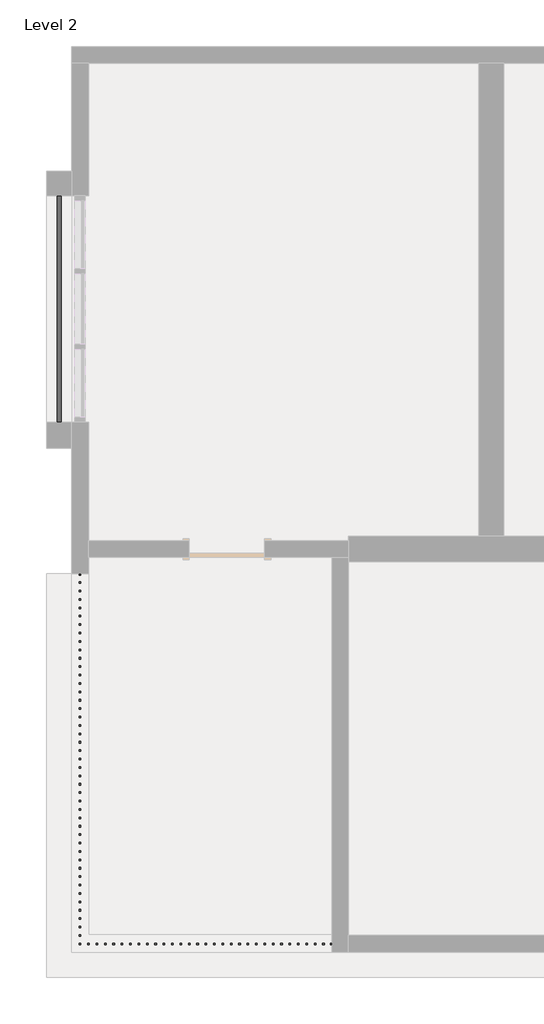
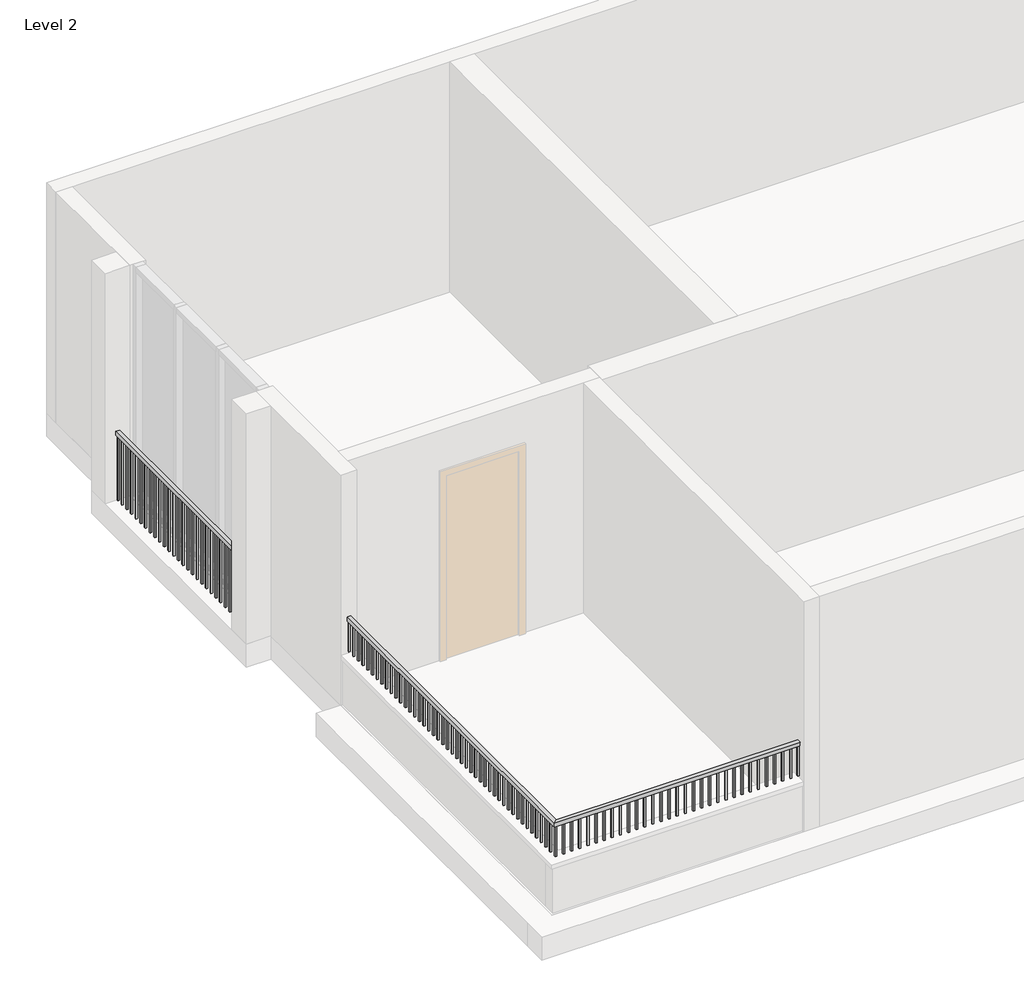
# One storey, part 2 of 2: 2 railings.
"""IFC4 building model written with IfcOpenShell, lengths in millimetres."""

from ifc_helpers import new_model, si_unit, frame, origin, place, context, project, spatial, polyline, outline, extrude, faceted_brep, element, save

model = new_model("IFC4")

# Units and contexts
model_context = context("Model", 3, world=origin())
ifc_project = project(units=[si_unit("LENGTHUNIT", "METRE", prefix="MILLI")], contexts=[model_context])

# Site, building, storey
site = spatial("IfcSite", under=ifc_project)
building = spatial("IfcBuilding", under=site)
storey = spatial("IfcBuildingStorey", under=building, Name="Level 2", Elevation=3048.0)

# Railings
placement = place(None, origin())
element("IfcRailing", 1, ObjectType="Handrail - Rectangular", at=placement, inside=storey, context=model_context, shape_type="SolidModel", body=[
    faceted_brep([(-15179.2169582, -9411.0617616, 4495.8), (-15179.2169582, -9411.0617616, 4445.0), (-15179.2169582, -9360.2617616, 4445.0), (-15179.2169582, -9360.2617616, 4495.8), (-18252.6169582, -9411.0617616, 4495.8), (-18252.6169582, -9411.0617616, 4445.0), (-18201.8169582, -9360.2617616, 4445.0), (-18201.8169582, -9360.2617616, 4495.8), (-18252.6169582, -4908.9117616, 4495.8), (-18201.8169582, -4908.9117616, 4495.8), (-18201.8169582, -4908.9117616, 4445.0), (-18252.6169582, -4908.9117616, 4445.0)], [[[0, 1, 2, 3]], [[1, 0, 4, 5]], [[2, 1, 5, 6]], [[3, 2, 6, 7]], [[0, 3, 7, 4]], [[8, 9, 10, 11]], [[5, 4, 8, 11]], [[6, 5, 11, 10]], [[7, 6, 10, 9]], [[4, 7, 9, 8]]]),
    extrude(outline(polyline([(-18217.6919582, -4924.7867616), (-18236.7419582, -4924.7867616), (-18236.7419582, -4905.7367616), (-18217.6919582, -4905.7367616), (-18217.6919582, -4924.7867616)])), frame((0.0, 0.0, 4038.6), z_axis=(0.0, 0.0, 1.0), x_axis=(1.0, 0.0, 0.0)), (0.0, 0.0, 1.0), 406.4),
    extrude(outline(polyline([(-18217.6919582, -5026.3867616), (-18236.7419582, -5026.3867616), (-18236.7419582, -5007.3367616), (-18217.6919582, -5007.3367616), (-18217.6919582, -5026.3867616)])), frame((0.0, 0.0, 4038.6), z_axis=(0.0, 0.0, 1.0), x_axis=(1.0, 0.0, 0.0)), (0.0, 0.0, 1.0), 406.4),
    extrude(outline(polyline([(-18217.6919582, -5127.9867616), (-18236.7419582, -5127.9867616), (-18236.7419582, -5108.9367616), (-18217.6919582, -5108.9367616), (-18217.6919582, -5127.9867616)])), frame((0.0, 0.0, 4038.6), z_axis=(0.0, 0.0, 1.0), x_axis=(1.0, 0.0, 0.0)), (0.0, 0.0, 1.0), 406.4),
    extrude(outline(polyline([(-18217.6919582, -5229.5867616), (-18236.7419582, -5229.5867616), (-18236.7419582, -5210.5367616), (-18217.6919582, -5210.5367616), (-18217.6919582, -5229.5867616)])), frame((0.0, 0.0, 4038.6), z_axis=(0.0, 0.0, 1.0), x_axis=(1.0, 0.0, 0.0)), (0.0, 0.0, 1.0), 406.4),
    extrude(outline(polyline([(-18217.6919582, -5331.1867616), (-18236.7419582, -5331.1867616), (-18236.7419582, -5312.1367616), (-18217.6919582, -5312.1367616), (-18217.6919582, -5331.1867616)])), frame((0.0, 0.0, 4038.6), z_axis=(0.0, 0.0, 1.0), x_axis=(1.0, 0.0, 0.0)), (0.0, 0.0, 1.0), 406.4),
    extrude(outline(polyline([(-18217.6919582, -5432.7867616), (-18236.7419582, -5432.7867616), (-18236.7419582, -5413.7367616), (-18217.6919582, -5413.7367616), (-18217.6919582, -5432.7867616)])), frame((0.0, 0.0, 4038.6), z_axis=(0.0, 0.0, 1.0), x_axis=(1.0, 0.0, 0.0)), (0.0, 0.0, 1.0), 406.4),
    extrude(outline(polyline([(-18217.6919582, -5534.3867616), (-18236.7419582, -5534.3867616), (-18236.7419582, -5515.3367616), (-18217.6919582, -5515.3367616), (-18217.6919582, -5534.3867616)])), frame((0.0, 0.0, 4038.6), z_axis=(0.0, 0.0, 1.0), x_axis=(1.0, 0.0, 0.0)), (0.0, 0.0, 1.0), 406.4),
    extrude(outline(polyline([(-18217.6919582, -5635.9867616), (-18236.7419582, -5635.9867616), (-18236.7419582, -5616.9367616), (-18217.6919582, -5616.9367616), (-18217.6919582, -5635.9867616)])), frame((0.0, 0.0, 4038.6), z_axis=(0.0, 0.0, 1.0), x_axis=(1.0, 0.0, 0.0)), (0.0, 0.0, 1.0), 406.4),
    extrude(outline(polyline([(-18217.6919582, -5737.5867616), (-18236.7419582, -5737.5867616), (-18236.7419582, -5718.5367616), (-18217.6919582, -5718.5367616), (-18217.6919582, -5737.5867616)])), frame((0.0, 0.0, 4038.6), z_axis=(0.0, 0.0, 1.0), x_axis=(1.0, 0.0, 0.0)), (0.0, 0.0, 1.0), 406.4),
    extrude(outline(polyline([(-18217.6919582, -5839.1867616), (-18236.7419582, -5839.1867616), (-18236.7419582, -5820.1367616), (-18217.6919582, -5820.1367616), (-18217.6919582, -5839.1867616)])), frame((0.0, 0.0, 4038.6), z_axis=(0.0, 0.0, 1.0), x_axis=(1.0, 0.0, 0.0)), (0.0, 0.0, 1.0), 406.4),
    extrude(outline(polyline([(-18217.6919582, -5940.7867616), (-18236.7419582, -5940.7867616), (-18236.7419582, -5921.7367616), (-18217.6919582, -5921.7367616), (-18217.6919582, -5940.7867616)])), frame((0.0, 0.0, 4038.6), z_axis=(0.0, 0.0, 1.0), x_axis=(1.0, 0.0, 0.0)), (0.0, 0.0, 1.0), 406.4),
    extrude(outline(polyline([(-18217.6919582, -6042.3867616), (-18236.7419582, -6042.3867616), (-18236.7419582, -6023.3367616), (-18217.6919582, -6023.3367616), (-18217.6919582, -6042.3867616)])), frame((0.0, 0.0, 4038.6), z_axis=(0.0, 0.0, 1.0), x_axis=(1.0, 0.0, 0.0)), (0.0, 0.0, 1.0), 406.4),
    extrude(outline(polyline([(-18217.6919582, -6143.9867616), (-18236.7419582, -6143.9867616), (-18236.7419582, -6124.9367616), (-18217.6919582, -6124.9367616), (-18217.6919582, -6143.9867616)])), frame((0.0, 0.0, 4038.6), z_axis=(0.0, 0.0, 1.0), x_axis=(1.0, 0.0, 0.0)), (0.0, 0.0, 1.0), 406.4),
    extrude(outline(polyline([(-18217.6919582, -6245.5867616), (-18236.7419582, -6245.5867616), (-18236.7419582, -6226.5367616), (-18217.6919582, -6226.5367616), (-18217.6919582, -6245.5867616)])), frame((0.0, 0.0, 4038.6), z_axis=(0.0, 0.0, 1.0), x_axis=(1.0, 0.0, 0.0)), (0.0, 0.0, 1.0), 406.4),
    extrude(outline(polyline([(-18217.6919582, -6347.1867616), (-18236.7419582, -6347.1867616), (-18236.7419582, -6328.1367616), (-18217.6919582, -6328.1367616), (-18217.6919582, -6347.1867616)])), frame((0.0, 0.0, 4038.6), z_axis=(0.0, 0.0, 1.0), x_axis=(1.0, 0.0, 0.0)), (0.0, 0.0, 1.0), 406.4),
    extrude(outline(polyline([(-18217.6919582, -6448.7867616), (-18236.7419582, -6448.7867616), (-18236.7419582, -6429.7367616), (-18217.6919582, -6429.7367616), (-18217.6919582, -6448.7867616)])), frame((0.0, 0.0, 4038.6), z_axis=(0.0, 0.0, 1.0), x_axis=(1.0, 0.0, 0.0)), (0.0, 0.0, 1.0), 406.4),
    extrude(outline(polyline([(-18217.6919582, -6550.3867616), (-18236.7419582, -6550.3867616), (-18236.7419582, -6531.3367616), (-18217.6919582, -6531.3367616), (-18217.6919582, -6550.3867616)])), frame((0.0, 0.0, 4038.6), z_axis=(0.0, 0.0, 1.0), x_axis=(1.0, 0.0, 0.0)), (0.0, 0.0, 1.0), 406.4),
    extrude(outline(polyline([(-18217.6919582, -6651.9867616), (-18236.7419582, -6651.9867616), (-18236.7419582, -6632.9367616), (-18217.6919582, -6632.9367616), (-18217.6919582, -6651.9867616)])), frame((0.0, 0.0, 4038.6), z_axis=(0.0, 0.0, 1.0), x_axis=(1.0, 0.0, 0.0)), (0.0, 0.0, 1.0), 406.4),
    extrude(outline(polyline([(-18217.6919582, -6753.5867616), (-18236.7419582, -6753.5867616), (-18236.7419582, -6734.5367616), (-18217.6919582, -6734.5367616), (-18217.6919582, -6753.5867616)])), frame((0.0, 0.0, 4038.6), z_axis=(0.0, 0.0, 1.0), x_axis=(1.0, 0.0, 0.0)), (0.0, 0.0, 1.0), 406.4),
    extrude(outline(polyline([(-18217.6919582, -6855.1867616), (-18236.7419582, -6855.1867616), (-18236.7419582, -6836.1367616), (-18217.6919582, -6836.1367616), (-18217.6919582, -6855.1867616)])), frame((0.0, 0.0, 4038.6), z_axis=(0.0, 0.0, 1.0), x_axis=(1.0, 0.0, 0.0)), (0.0, 0.0, 1.0), 406.4),
    extrude(outline(polyline([(-18217.6919582, -6956.7867616), (-18236.7419582, -6956.7867616), (-18236.7419582, -6937.7367616), (-18217.6919582, -6937.7367616), (-18217.6919582, -6956.7867616)])), frame((0.0, 0.0, 4038.6), z_axis=(0.0, 0.0, 1.0), x_axis=(1.0, 0.0, 0.0)), (0.0, 0.0, 1.0), 406.4),
    extrude(outline(polyline([(-18217.6919582, -7058.3867616), (-18236.7419582, -7058.3867616), (-18236.7419582, -7039.3367616), (-18217.6919582, -7039.3367616), (-18217.6919582, -7058.3867616)])), frame((0.0, 0.0, 4038.6), z_axis=(0.0, 0.0, 1.0), x_axis=(1.0, 0.0, 0.0)), (0.0, 0.0, 1.0), 406.4),
    extrude(outline(polyline([(-18217.6919582, -7159.9867616), (-18236.7419582, -7159.9867616), (-18236.7419582, -7140.9367616), (-18217.6919582, -7140.9367616), (-18217.6919582, -7159.9867616)])), frame((0.0, 0.0, 4038.6), z_axis=(0.0, 0.0, 1.0), x_axis=(1.0, 0.0, 0.0)), (0.0, 0.0, 1.0), 406.4),
    extrude(outline(polyline([(-18217.6919582, -7261.5867616), (-18236.7419582, -7261.5867616), (-18236.7419582, -7242.5367616), (-18217.6919582, -7242.5367616), (-18217.6919582, -7261.5867616)])), frame((0.0, 0.0, 4038.6), z_axis=(0.0, 0.0, 1.0), x_axis=(1.0, 0.0, 0.0)), (0.0, 0.0, 1.0), 406.4),
    extrude(outline(polyline([(-18217.6919582, -7363.1867616), (-18236.7419582, -7363.1867616), (-18236.7419582, -7344.1367616), (-18217.6919582, -7344.1367616), (-18217.6919582, -7363.1867616)])), frame((0.0, 0.0, 4038.6), z_axis=(0.0, 0.0, 1.0), x_axis=(1.0, 0.0, 0.0)), (0.0, 0.0, 1.0), 406.4),
    extrude(outline(polyline([(-18217.6919582, -7464.7867616), (-18236.7419582, -7464.7867616), (-18236.7419582, -7445.7367616), (-18217.6919582, -7445.7367616), (-18217.6919582, -7464.7867616)])), frame((0.0, 0.0, 4038.6), z_axis=(0.0, 0.0, 1.0), x_axis=(1.0, 0.0, 0.0)), (0.0, 0.0, 1.0), 406.4),
    extrude(outline(polyline([(-18217.6919582, -7566.3867616), (-18236.7419582, -7566.3867616), (-18236.7419582, -7547.3367616), (-18217.6919582, -7547.3367616), (-18217.6919582, -7566.3867616)])), frame((0.0, 0.0, 4038.6), z_axis=(0.0, 0.0, 1.0), x_axis=(1.0, 0.0, 0.0)), (0.0, 0.0, 1.0), 406.4),
    extrude(outline(polyline([(-18217.6919582, -7667.9867616), (-18236.7419582, -7667.9867616), (-18236.7419582, -7648.9367616), (-18217.6919582, -7648.9367616), (-18217.6919582, -7667.9867616)])), frame((0.0, 0.0, 4038.6), z_axis=(0.0, 0.0, 1.0), x_axis=(1.0, 0.0, 0.0)), (0.0, 0.0, 1.0), 406.4),
    extrude(outline(polyline([(-18217.6919582, -7769.5867616), (-18236.7419582, -7769.5867616), (-18236.7419582, -7750.5367616), (-18217.6919582, -7750.5367616), (-18217.6919582, -7769.5867616)])), frame((0.0, 0.0, 4038.6), z_axis=(0.0, 0.0, 1.0), x_axis=(1.0, 0.0, 0.0)), (0.0, 0.0, 1.0), 406.4),
    extrude(outline(polyline([(-18217.6919582, -7871.1867616), (-18236.7419582, -7871.1867616), (-18236.7419582, -7852.1367616), (-18217.6919582, -7852.1367616), (-18217.6919582, -7871.1867616)])), frame((0.0, 0.0, 4038.6), z_axis=(0.0, 0.0, 1.0), x_axis=(1.0, 0.0, 0.0)), (0.0, 0.0, 1.0), 406.4),
    extrude(outline(polyline([(-18217.6919582, -7972.7867616), (-18236.7419582, -7972.7867616), (-18236.7419582, -7953.7367616), (-18217.6919582, -7953.7367616), (-18217.6919582, -7972.7867616)])), frame((0.0, 0.0, 4038.6), z_axis=(0.0, 0.0, 1.0), x_axis=(1.0, 0.0, 0.0)), (0.0, 0.0, 1.0), 406.4),
    extrude(outline(polyline([(-18217.6919582, -8074.3867616), (-18236.7419582, -8074.3867616), (-18236.7419582, -8055.3367616), (-18217.6919582, -8055.3367616), (-18217.6919582, -8074.3867616)])), frame((0.0, 0.0, 4038.6), z_axis=(0.0, 0.0, 1.0), x_axis=(1.0, 0.0, 0.0)), (0.0, 0.0, 1.0), 406.4),
    extrude(outline(polyline([(-18217.6919582, -8175.9867616), (-18236.7419582, -8175.9867616), (-18236.7419582, -8156.9367616), (-18217.6919582, -8156.9367616), (-18217.6919582, -8175.9867616)])), frame((0.0, 0.0, 4038.6), z_axis=(0.0, 0.0, 1.0), x_axis=(1.0, 0.0, 0.0)), (0.0, 0.0, 1.0), 406.4),
    extrude(outline(polyline([(-18217.6919582, -8277.5867616), (-18236.7419582, -8277.5867616), (-18236.7419582, -8258.5367616), (-18217.6919582, -8258.5367616), (-18217.6919582, -8277.5867616)])), frame((0.0, 0.0, 4038.6), z_axis=(0.0, 0.0, 1.0), x_axis=(1.0, 0.0, 0.0)), (0.0, 0.0, 1.0), 406.4),
    extrude(outline(polyline([(-18217.6919582, -8379.1867616), (-18236.7419582, -8379.1867616), (-18236.7419582, -8360.1367616), (-18217.6919582, -8360.1367616), (-18217.6919582, -8379.1867616)])), frame((0.0, 0.0, 4038.6), z_axis=(0.0, 0.0, 1.0), x_axis=(1.0, 0.0, 0.0)), (0.0, 0.0, 1.0), 406.4),
    extrude(outline(polyline([(-18217.6919582, -8480.7867616), (-18236.7419582, -8480.7867616), (-18236.7419582, -8461.7367616), (-18217.6919582, -8461.7367616), (-18217.6919582, -8480.7867616)])), frame((0.0, 0.0, 4038.6), z_axis=(0.0, 0.0, 1.0), x_axis=(1.0, 0.0, 0.0)), (0.0, 0.0, 1.0), 406.4),
    extrude(outline(polyline([(-18217.6919582, -8582.3867616), (-18236.7419582, -8582.3867616), (-18236.7419582, -8563.3367616), (-18217.6919582, -8563.3367616), (-18217.6919582, -8582.3867616)])), frame((0.0, 0.0, 4038.6), z_axis=(0.0, 0.0, 1.0), x_axis=(1.0, 0.0, 0.0)), (0.0, 0.0, 1.0), 406.4),
    extrude(outline(polyline([(-18217.6919582, -8683.9867616), (-18236.7419582, -8683.9867616), (-18236.7419582, -8664.9367616), (-18217.6919582, -8664.9367616), (-18217.6919582, -8683.9867616)])), frame((0.0, 0.0, 4038.6), z_axis=(0.0, 0.0, 1.0), x_axis=(1.0, 0.0, 0.0)), (0.0, 0.0, 1.0), 406.4),
    extrude(outline(polyline([(-18217.6919582, -8785.5867616), (-18236.7419582, -8785.5867616), (-18236.7419582, -8766.5367616), (-18217.6919582, -8766.5367616), (-18217.6919582, -8785.5867616)])), frame((0.0, 0.0, 4038.6), z_axis=(0.0, 0.0, 1.0), x_axis=(1.0, 0.0, 0.0)), (0.0, 0.0, 1.0), 406.4),
    extrude(outline(polyline([(-18217.6919582, -8887.1867616), (-18236.7419582, -8887.1867616), (-18236.7419582, -8868.1367616), (-18217.6919582, -8868.1367616), (-18217.6919582, -8887.1867616)])), frame((0.0, 0.0, 4038.6), z_axis=(0.0, 0.0, 1.0), x_axis=(1.0, 0.0, 0.0)), (0.0, 0.0, 1.0), 406.4),
    extrude(outline(polyline([(-18217.6919582, -8988.7867616), (-18236.7419582, -8988.7867616), (-18236.7419582, -8969.7367616), (-18217.6919582, -8969.7367616), (-18217.6919582, -8988.7867616)])), frame((0.0, 0.0, 4038.6), z_axis=(0.0, 0.0, 1.0), x_axis=(1.0, 0.0, 0.0)), (0.0, 0.0, 1.0), 406.4),
    extrude(outline(polyline([(-18217.6919582, -9090.3867616), (-18236.7419582, -9090.3867616), (-18236.7419582, -9071.3367616), (-18217.6919582, -9071.3367616), (-18217.6919582, -9090.3867616)])), frame((0.0, 0.0, 4038.6), z_axis=(0.0, 0.0, 1.0), x_axis=(1.0, 0.0, 0.0)), (0.0, 0.0, 1.0), 406.4),
    extrude(outline(polyline([(-18217.6919582, -9191.9867616), (-18236.7419582, -9191.9867616), (-18236.7419582, -9172.9367616), (-18217.6919582, -9172.9367616), (-18217.6919582, -9191.9867616)])), frame((0.0, 0.0, 4038.6), z_axis=(0.0, 0.0, 1.0), x_axis=(1.0, 0.0, 0.0)), (0.0, 0.0, 1.0), 406.4),
    extrude(outline(polyline([(-18217.6919582, -9293.5867616), (-18236.7419582, -9293.5867616), (-18236.7419582, -9274.5367616), (-18217.6919582, -9274.5367616), (-18217.6919582, -9293.5867616)])), frame((0.0, 0.0, 4038.6), z_axis=(0.0, 0.0, 1.0), x_axis=(1.0, 0.0, 0.0)), (0.0, 0.0, 1.0), 406.4),
    extrude(outline(polyline([(-18116.0919582, -9376.1367616), (-18116.0919582, -9395.1867616), (-18135.1419582, -9395.1867616), (-18135.1419582, -9376.1367616), (-18116.0919582, -9376.1367616)])), frame((0.0, 0.0, 4038.6), z_axis=(0.0, 0.0, 1.0), x_axis=(1.0, 0.0, 0.0)), (0.0, 0.0, 1.0), 406.4),
    extrude(outline(polyline([(-18014.4919582, -9376.1367616), (-18014.4919582, -9395.1867616), (-18033.5419582, -9395.1867616), (-18033.5419582, -9376.1367616), (-18014.4919582, -9376.1367616)])), frame((0.0, 0.0, 4038.6), z_axis=(0.0, 0.0, 1.0), x_axis=(1.0, 0.0, 0.0)), (0.0, 0.0, 1.0), 406.4),
    extrude(outline(polyline([(-17912.8919582, -9376.1367616), (-17912.8919582, -9395.1867616), (-17931.9419582, -9395.1867616), (-17931.9419582, -9376.1367616), (-17912.8919582, -9376.1367616)])), frame((0.0, 0.0, 4038.6), z_axis=(0.0, 0.0, 1.0), x_axis=(1.0, 0.0, 0.0)), (0.0, 0.0, 1.0), 406.4),
    extrude(outline(polyline([(-17811.2919582, -9376.1367616), (-17811.2919582, -9395.1867616), (-17830.3419582, -9395.1867616), (-17830.3419582, -9376.1367616), (-17811.2919582, -9376.1367616)])), frame((0.0, 0.0, 4038.6), z_axis=(0.0, 0.0, 1.0), x_axis=(1.0, 0.0, 0.0)), (0.0, 0.0, 1.0), 406.4),
    extrude(outline(polyline([(-17709.6919582, -9376.1367616), (-17709.6919582, -9395.1867616), (-17728.7419582, -9395.1867616), (-17728.7419582, -9376.1367616), (-17709.6919582, -9376.1367616)])), frame((0.0, 0.0, 4038.6), z_axis=(0.0, 0.0, 1.0), x_axis=(1.0, 0.0, 0.0)), (0.0, 0.0, 1.0), 406.4),
    extrude(outline(polyline([(-17608.0919582, -9376.1367616), (-17608.0919582, -9395.1867616), (-17627.1419582, -9395.1867616), (-17627.1419582, -9376.1367616), (-17608.0919582, -9376.1367616)])), frame((0.0, 0.0, 4038.6), z_axis=(0.0, 0.0, 1.0), x_axis=(1.0, 0.0, 0.0)), (0.0, 0.0, 1.0), 406.4),
    extrude(outline(polyline([(-17506.4919582, -9376.1367616), (-17506.4919582, -9395.1867616), (-17525.5419582, -9395.1867616), (-17525.5419582, -9376.1367616), (-17506.4919582, -9376.1367616)])), frame((0.0, 0.0, 4038.6), z_axis=(0.0, 0.0, 1.0), x_axis=(1.0, 0.0, 0.0)), (0.0, 0.0, 1.0), 406.4),
    extrude(outline(polyline([(-17404.8919582, -9376.1367616), (-17404.8919582, -9395.1867616), (-17423.9419582, -9395.1867616), (-17423.9419582, -9376.1367616), (-17404.8919582, -9376.1367616)])), frame((0.0, 0.0, 4038.6), z_axis=(0.0, 0.0, 1.0), x_axis=(1.0, 0.0, 0.0)), (0.0, 0.0, 1.0), 406.4),
    extrude(outline(polyline([(-17303.2919582, -9376.1367616), (-17303.2919582, -9395.1867616), (-17322.3419582, -9395.1867616), (-17322.3419582, -9376.1367616), (-17303.2919582, -9376.1367616)])), frame((0.0, 0.0, 4038.6), z_axis=(0.0, 0.0, 1.0), x_axis=(1.0, 0.0, 0.0)), (0.0, 0.0, 1.0), 406.4),
    extrude(outline(polyline([(-17201.6919582, -9376.1367616), (-17201.6919582, -9395.1867616), (-17220.7419582, -9395.1867616), (-17220.7419582, -9376.1367616), (-17201.6919582, -9376.1367616)])), frame((0.0, 0.0, 4038.6), z_axis=(0.0, 0.0, 1.0), x_axis=(1.0, 0.0, 0.0)), (0.0, 0.0, 1.0), 406.4),
    extrude(outline(polyline([(-17100.0919582, -9376.1367616), (-17100.0919582, -9395.1867616), (-17119.1419582, -9395.1867616), (-17119.1419582, -9376.1367616), (-17100.0919582, -9376.1367616)])), frame((0.0, 0.0, 4038.6), z_axis=(0.0, 0.0, 1.0), x_axis=(1.0, 0.0, 0.0)), (0.0, 0.0, 1.0), 406.4),
    extrude(outline(polyline([(-16998.4919582, -9376.1367616), (-16998.4919582, -9395.1867616), (-17017.5419582, -9395.1867616), (-17017.5419582, -9376.1367616), (-16998.4919582, -9376.1367616)])), frame((0.0, 0.0, 4038.6), z_axis=(0.0, 0.0, 1.0), x_axis=(1.0, 0.0, 0.0)), (0.0, 0.0, 1.0), 406.4),
    extrude(outline(polyline([(-16896.8919582, -9376.1367616), (-16896.8919582, -9395.1867616), (-16915.9419582, -9395.1867616), (-16915.9419582, -9376.1367616), (-16896.8919582, -9376.1367616)])), frame((0.0, 0.0, 4038.6), z_axis=(0.0, 0.0, 1.0), x_axis=(1.0, 0.0, 0.0)), (0.0, 0.0, 1.0), 406.4),
    extrude(outline(polyline([(-16795.2919582, -9376.1367616), (-16795.2919582, -9395.1867616), (-16814.3419582, -9395.1867616), (-16814.3419582, -9376.1367616), (-16795.2919582, -9376.1367616)])), frame((0.0, 0.0, 4038.6), z_axis=(0.0, 0.0, 1.0), x_axis=(1.0, 0.0, 0.0)), (0.0, 0.0, 1.0), 406.4),
    extrude(outline(polyline([(-16693.6919582, -9376.1367616), (-16693.6919582, -9395.1867616), (-16712.7419582, -9395.1867616), (-16712.7419582, -9376.1367616), (-16693.6919582, -9376.1367616)])), frame((0.0, 0.0, 4038.6), z_axis=(0.0, 0.0, 1.0), x_axis=(1.0, 0.0, 0.0)), (0.0, 0.0, 1.0), 406.4),
    extrude(outline(polyline([(-16592.0919582, -9376.1367616), (-16592.0919582, -9395.1867616), (-16611.1419582, -9395.1867616), (-16611.1419582, -9376.1367616), (-16592.0919582, -9376.1367616)])), frame((0.0, 0.0, 4038.6), z_axis=(0.0, 0.0, 1.0), x_axis=(1.0, 0.0, 0.0)), (0.0, 0.0, 1.0), 406.4),
    extrude(outline(polyline([(-16490.4919582, -9376.1367616), (-16490.4919582, -9395.1867616), (-16509.5419582, -9395.1867616), (-16509.5419582, -9376.1367616), (-16490.4919582, -9376.1367616)])), frame((0.0, 0.0, 4038.6), z_axis=(0.0, 0.0, 1.0), x_axis=(1.0, 0.0, 0.0)), (0.0, 0.0, 1.0), 406.4),
    extrude(outline(polyline([(-16388.8919582, -9376.1367616), (-16388.8919582, -9395.1867616), (-16407.9419582, -9395.1867616), (-16407.9419582, -9376.1367616), (-16388.8919582, -9376.1367616)])), frame((0.0, 0.0, 4038.6), z_axis=(0.0, 0.0, 1.0), x_axis=(1.0, 0.0, 0.0)), (0.0, 0.0, 1.0), 406.4),
    extrude(outline(polyline([(-16287.2919582, -9376.1367616), (-16287.2919582, -9395.1867616), (-16306.3419582, -9395.1867616), (-16306.3419582, -9376.1367616), (-16287.2919582, -9376.1367616)])), frame((0.0, 0.0, 4038.6), z_axis=(0.0, 0.0, 1.0), x_axis=(1.0, 0.0, 0.0)), (0.0, 0.0, 1.0), 406.4),
    extrude(outline(polyline([(-16185.6919582, -9376.1367616), (-16185.6919582, -9395.1867616), (-16204.7419582, -9395.1867616), (-16204.7419582, -9376.1367616), (-16185.6919582, -9376.1367616)])), frame((0.0, 0.0, 4038.6), z_axis=(0.0, 0.0, 1.0), x_axis=(1.0, 0.0, 0.0)), (0.0, 0.0, 1.0), 406.4),
    extrude(outline(polyline([(-16084.0919582, -9376.1367616), (-16084.0919582, -9395.1867616), (-16103.1419582, -9395.1867616), (-16103.1419582, -9376.1367616), (-16084.0919582, -9376.1367616)])), frame((0.0, 0.0, 4038.6), z_axis=(0.0, 0.0, 1.0), x_axis=(1.0, 0.0, 0.0)), (0.0, 0.0, 1.0), 406.4),
    extrude(outline(polyline([(-15982.4919582, -9376.1367616), (-15982.4919582, -9395.1867616), (-16001.5419582, -9395.1867616), (-16001.5419582, -9376.1367616), (-15982.4919582, -9376.1367616)])), frame((0.0, 0.0, 4038.6), z_axis=(0.0, 0.0, 1.0), x_axis=(1.0, 0.0, 0.0)), (0.0, 0.0, 1.0), 406.4),
    extrude(outline(polyline([(-15880.8919582, -9376.1367616), (-15880.8919582, -9395.1867616), (-15899.9419582, -9395.1867616), (-15899.9419582, -9376.1367616), (-15880.8919582, -9376.1367616)])), frame((0.0, 0.0, 4038.6), z_axis=(0.0, 0.0, 1.0), x_axis=(1.0, 0.0, 0.0)), (0.0, 0.0, 1.0), 406.4),
    extrude(outline(polyline([(-15779.2919582, -9376.1367616), (-15779.2919582, -9395.1867616), (-15798.3419582, -9395.1867616), (-15798.3419582, -9376.1367616), (-15779.2919582, -9376.1367616)])), frame((0.0, 0.0, 4038.6), z_axis=(0.0, 0.0, 1.0), x_axis=(1.0, 0.0, 0.0)), (0.0, 0.0, 1.0), 406.4),
    extrude(outline(polyline([(-15677.6919582, -9376.1367616), (-15677.6919582, -9395.1867616), (-15696.7419582, -9395.1867616), (-15696.7419582, -9376.1367616), (-15677.6919582, -9376.1367616)])), frame((0.0, 0.0, 4038.6), z_axis=(0.0, 0.0, 1.0), x_axis=(1.0, 0.0, 0.0)), (0.0, 0.0, 1.0), 406.4),
    extrude(outline(polyline([(-15576.0919582, -9376.1367616), (-15576.0919582, -9395.1867616), (-15595.1419582, -9395.1867616), (-15595.1419582, -9376.1367616), (-15576.0919582, -9376.1367616)])), frame((0.0, 0.0, 4038.6), z_axis=(0.0, 0.0, 1.0), x_axis=(1.0, 0.0, 0.0)), (0.0, 0.0, 1.0), 406.4),
    extrude(outline(polyline([(-15474.4919582, -9376.1367616), (-15474.4919582, -9395.1867616), (-15493.5419582, -9395.1867616), (-15493.5419582, -9376.1367616), (-15474.4919582, -9376.1367616)])), frame((0.0, 0.0, 4038.6), z_axis=(0.0, 0.0, 1.0), x_axis=(1.0, 0.0, 0.0)), (0.0, 0.0, 1.0), 406.4),
    extrude(outline(polyline([(-15372.8919582, -9376.1367616), (-15372.8919582, -9395.1867616), (-15391.9419582, -9395.1867616), (-15391.9419582, -9376.1367616), (-15372.8919582, -9376.1367616)])), frame((0.0, 0.0, 4038.6), z_axis=(0.0, 0.0, 1.0), x_axis=(1.0, 0.0, 0.0)), (0.0, 0.0, 1.0), 406.4),
    extrude(outline(polyline([(-15271.2919582, -9376.1367616), (-15271.2919582, -9395.1867616), (-15290.3419582, -9395.1867616), (-15290.3419582, -9376.1367616), (-15271.2919582, -9376.1367616)])), frame((0.0, 0.0, 4038.6), z_axis=(0.0, 0.0, 1.0), x_axis=(1.0, 0.0, 0.0)), (0.0, 0.0, 1.0), 406.4),
    extrude(outline(polyline([(-18217.6919582, -9376.1367616), (-18217.6919582, -9395.1867616), (-18236.7419582, -9395.1867616), (-18236.7419582, -9376.1367616), (-18217.6919582, -9376.1367616)])), frame((0.0, 0.0, 4038.6), z_axis=(0.0, 0.0, 1.0), x_axis=(1.0, 0.0, 0.0)), (0.0, 0.0, 1.0), 406.4),
    extrude(outline(polyline([(-18217.6919582, -4927.9617616), (-18236.7419582, -4927.9617616), (-18236.7419582, -4908.9117616), (-18217.6919582, -4908.9117616), (-18217.6919582, -4927.9617616)])), frame((0.0, 0.0, 4038.6), z_axis=(0.0, 0.0, 1.0), x_axis=(1.0, 0.0, 0.0)), (0.0, 0.0, 1.0), 406.4),
    extrude(outline(polyline([(-15179.2169582, -9376.1367616), (-15179.2169582, -9395.1867616), (-15198.2669582, -9395.1867616), (-15198.2669582, -9376.1367616), (-15179.2169582, -9376.1367616)])), frame((0.0, 0.0, 4038.6), z_axis=(0.0, 0.0, 1.0), x_axis=(1.0, 0.0, 0.0)), (0.0, 0.0, 1.0), 406.4),
])
element("IfcRailing", 2, ObjectType="Handrail - Rectangular 2", at=placement, inside=storey, context=model_context, shape_type="SweptSolid", body=[
    extrude(outline(polyline([(-18506.6169582, -336.9117616), (-18455.8169582, -336.9117616), (-18455.8169582, -3080.1117616), (-18506.6169582, -3080.1117616), (-18506.6169582, -336.9117616)])), frame((0.0, 0.0, 4216.4), z_axis=(0.0, 0.0, 1.0), x_axis=(1.0, 0.0, 0.0)), (0.0, 0.0, 1.0), 50.8),
    extrude(outline(polyline([(-18490.7419582, -2968.9867616), (-18471.6919582, -2968.9867616), (-18471.6919582, -2988.0367616), (-18490.7419582, -2988.0367616), (-18490.7419582, -2968.9867616)])), frame((0.0, 0.0, 3352.8), z_axis=(0.0, 0.0, 1.0), x_axis=(1.0, 0.0, 0.0)), (0.0, 0.0, 1.0), 863.6),
    extrude(outline(polyline([(-18490.7419582, -2867.3867616), (-18471.6919582, -2867.3867616), (-18471.6919582, -2886.4367616), (-18490.7419582, -2886.4367616), (-18490.7419582, -2867.3867616)])), frame((0.0, 0.0, 3352.8), z_axis=(0.0, 0.0, 1.0), x_axis=(1.0, 0.0, 0.0)), (0.0, 0.0, 1.0), 863.6),
    extrude(outline(polyline([(-18490.7419582, -2765.7867616), (-18471.6919582, -2765.7867616), (-18471.6919582, -2784.8367616), (-18490.7419582, -2784.8367616), (-18490.7419582, -2765.7867616)])), frame((0.0, 0.0, 3352.8), z_axis=(0.0, 0.0, 1.0), x_axis=(1.0, 0.0, 0.0)), (0.0, 0.0, 1.0), 863.6),
    extrude(outline(polyline([(-18490.7419582, -2664.1867616), (-18471.6919582, -2664.1867616), (-18471.6919582, -2683.2367616), (-18490.7419582, -2683.2367616), (-18490.7419582, -2664.1867616)])), frame((0.0, 0.0, 3352.8), z_axis=(0.0, 0.0, 1.0), x_axis=(1.0, 0.0, 0.0)), (0.0, 0.0, 1.0), 863.6),
    extrude(outline(polyline([(-18490.7419582, -2562.5867616), (-18471.6919582, -2562.5867616), (-18471.6919582, -2581.6367616), (-18490.7419582, -2581.6367616), (-18490.7419582, -2562.5867616)])), frame((0.0, 0.0, 3352.8), z_axis=(0.0, 0.0, 1.0), x_axis=(1.0, 0.0, 0.0)), (0.0, 0.0, 1.0), 863.6),
    extrude(outline(polyline([(-18490.7419582, -2460.9867616), (-18471.6919582, -2460.9867616), (-18471.6919582, -2480.0367616), (-18490.7419582, -2480.0367616), (-18490.7419582, -2460.9867616)])), frame((0.0, 0.0, 3352.8), z_axis=(0.0, 0.0, 1.0), x_axis=(1.0, 0.0, 0.0)), (0.0, 0.0, 1.0), 863.6),
    extrude(outline(polyline([(-18490.7419582, -2359.3867616), (-18471.6919582, -2359.3867616), (-18471.6919582, -2378.4367616), (-18490.7419582, -2378.4367616), (-18490.7419582, -2359.3867616)])), frame((0.0, 0.0, 3352.8), z_axis=(0.0, 0.0, 1.0), x_axis=(1.0, 0.0, 0.0)), (0.0, 0.0, 1.0), 863.6),
    extrude(outline(polyline([(-18490.7419582, -2257.7867616), (-18471.6919582, -2257.7867616), (-18471.6919582, -2276.8367616), (-18490.7419582, -2276.8367616), (-18490.7419582, -2257.7867616)])), frame((0.0, 0.0, 3352.8), z_axis=(0.0, 0.0, 1.0), x_axis=(1.0, 0.0, 0.0)), (0.0, 0.0, 1.0), 863.6),
    extrude(outline(polyline([(-18490.7419582, -2156.1867616), (-18471.6919582, -2156.1867616), (-18471.6919582, -2175.2367616), (-18490.7419582, -2175.2367616), (-18490.7419582, -2156.1867616)])), frame((0.0, 0.0, 3352.8), z_axis=(0.0, 0.0, 1.0), x_axis=(1.0, 0.0, 0.0)), (0.0, 0.0, 1.0), 863.6),
    extrude(outline(polyline([(-18490.7419582, -2054.5867616), (-18471.6919582, -2054.5867616), (-18471.6919582, -2073.6367616), (-18490.7419582, -2073.6367616), (-18490.7419582, -2054.5867616)])), frame((0.0, 0.0, 3352.8), z_axis=(0.0, 0.0, 1.0), x_axis=(1.0, 0.0, 0.0)), (0.0, 0.0, 1.0), 863.6),
    extrude(outline(polyline([(-18490.7419582, -1952.9867616), (-18471.6919582, -1952.9867616), (-18471.6919582, -1972.0367616), (-18490.7419582, -1972.0367616), (-18490.7419582, -1952.9867616)])), frame((0.0, 0.0, 3352.8), z_axis=(0.0, 0.0, 1.0), x_axis=(1.0, 0.0, 0.0)), (0.0, 0.0, 1.0), 863.6),
    extrude(outline(polyline([(-18490.7419582, -1851.3867616), (-18471.6919582, -1851.3867616), (-18471.6919582, -1870.4367616), (-18490.7419582, -1870.4367616), (-18490.7419582, -1851.3867616)])), frame((0.0, 0.0, 3352.8), z_axis=(0.0, 0.0, 1.0), x_axis=(1.0, 0.0, 0.0)), (0.0, 0.0, 1.0), 863.6),
    extrude(outline(polyline([(-18490.7419582, -1749.7867616), (-18471.6919582, -1749.7867616), (-18471.6919582, -1768.8367616), (-18490.7419582, -1768.8367616), (-18490.7419582, -1749.7867616)])), frame((0.0, 0.0, 3352.8), z_axis=(0.0, 0.0, 1.0), x_axis=(1.0, 0.0, 0.0)), (0.0, 0.0, 1.0), 863.6),
    extrude(outline(polyline([(-18490.7419582, -1648.1867616), (-18471.6919582, -1648.1867616), (-18471.6919582, -1667.2367616), (-18490.7419582, -1667.2367616), (-18490.7419582, -1648.1867616)])), frame((0.0, 0.0, 3352.8), z_axis=(0.0, 0.0, 1.0), x_axis=(1.0, 0.0, 0.0)), (0.0, 0.0, 1.0), 863.6),
    extrude(outline(polyline([(-18490.7419582, -1546.5867616), (-18471.6919582, -1546.5867616), (-18471.6919582, -1565.6367616), (-18490.7419582, -1565.6367616), (-18490.7419582, -1546.5867616)])), frame((0.0, 0.0, 3352.8), z_axis=(0.0, 0.0, 1.0), x_axis=(1.0, 0.0, 0.0)), (0.0, 0.0, 1.0), 863.6),
    extrude(outline(polyline([(-18490.7419582, -1444.9867616), (-18471.6919582, -1444.9867616), (-18471.6919582, -1464.0367616), (-18490.7419582, -1464.0367616), (-18490.7419582, -1444.9867616)])), frame((0.0, 0.0, 3352.8), z_axis=(0.0, 0.0, 1.0), x_axis=(1.0, 0.0, 0.0)), (0.0, 0.0, 1.0), 863.6),
    extrude(outline(polyline([(-18490.7419582, -1343.3867616), (-18471.6919582, -1343.3867616), (-18471.6919582, -1362.4367616), (-18490.7419582, -1362.4367616), (-18490.7419582, -1343.3867616)])), frame((0.0, 0.0, 3352.8), z_axis=(0.0, 0.0, 1.0), x_axis=(1.0, 0.0, 0.0)), (0.0, 0.0, 1.0), 863.6),
    extrude(outline(polyline([(-18490.7419582, -1241.7867616), (-18471.6919582, -1241.7867616), (-18471.6919582, -1260.8367616), (-18490.7419582, -1260.8367616), (-18490.7419582, -1241.7867616)])), frame((0.0, 0.0, 3352.8), z_axis=(0.0, 0.0, 1.0), x_axis=(1.0, 0.0, 0.0)), (0.0, 0.0, 1.0), 863.6),
    extrude(outline(polyline([(-18490.7419582, -1140.1867616), (-18471.6919582, -1140.1867616), (-18471.6919582, -1159.2367616), (-18490.7419582, -1159.2367616), (-18490.7419582, -1140.1867616)])), frame((0.0, 0.0, 3352.8), z_axis=(0.0, 0.0, 1.0), x_axis=(1.0, 0.0, 0.0)), (0.0, 0.0, 1.0), 863.6),
    extrude(outline(polyline([(-18490.7419582, -1038.5867616), (-18471.6919582, -1038.5867616), (-18471.6919582, -1057.6367616), (-18490.7419582, -1057.6367616), (-18490.7419582, -1038.5867616)])), frame((0.0, 0.0, 3352.8), z_axis=(0.0, 0.0, 1.0), x_axis=(1.0, 0.0, 0.0)), (0.0, 0.0, 1.0), 863.6),
    extrude(outline(polyline([(-18490.7419582, -936.9867616), (-18471.6919582, -936.9867616), (-18471.6919582, -956.0367616), (-18490.7419582, -956.0367616), (-18490.7419582, -936.9867616)])), frame((0.0, 0.0, 3352.8), z_axis=(0.0, 0.0, 1.0), x_axis=(1.0, 0.0, 0.0)), (0.0, 0.0, 1.0), 863.6),
    extrude(outline(polyline([(-18490.7419582, -835.3867616), (-18471.6919582, -835.3867616), (-18471.6919582, -854.4367616), (-18490.7419582, -854.4367616), (-18490.7419582, -835.3867616)])), frame((0.0, 0.0, 3352.8), z_axis=(0.0, 0.0, 1.0), x_axis=(1.0, 0.0, 0.0)), (0.0, 0.0, 1.0), 863.6),
    extrude(outline(polyline([(-18490.7419582, -733.7867616), (-18471.6919582, -733.7867616), (-18471.6919582, -752.8367616), (-18490.7419582, -752.8367616), (-18490.7419582, -733.7867616)])), frame((0.0, 0.0, 3352.8), z_axis=(0.0, 0.0, 1.0), x_axis=(1.0, 0.0, 0.0)), (0.0, 0.0, 1.0), 863.6),
    extrude(outline(polyline([(-18490.7419582, -632.1867616), (-18471.6919582, -632.1867616), (-18471.6919582, -651.2367616), (-18490.7419582, -651.2367616), (-18490.7419582, -632.1867616)])), frame((0.0, 0.0, 3352.8), z_axis=(0.0, 0.0, 1.0), x_axis=(1.0, 0.0, 0.0)), (0.0, 0.0, 1.0), 863.6),
    extrude(outline(polyline([(-18490.7419582, -530.5867616), (-18471.6919582, -530.5867616), (-18471.6919582, -549.6367616), (-18490.7419582, -549.6367616), (-18490.7419582, -530.5867616)])), frame((0.0, 0.0, 3352.8), z_axis=(0.0, 0.0, 1.0), x_axis=(1.0, 0.0, 0.0)), (0.0, 0.0, 1.0), 863.6),
    extrude(outline(polyline([(-18490.7419582, -428.9867616), (-18471.6919582, -428.9867616), (-18471.6919582, -448.0367616), (-18490.7419582, -448.0367616), (-18490.7419582, -428.9867616)])), frame((0.0, 0.0, 3352.8), z_axis=(0.0, 0.0, 1.0), x_axis=(1.0, 0.0, 0.0)), (0.0, 0.0, 1.0), 863.6),
    extrude(outline(polyline([(-18490.7419582, -3061.0617616), (-18471.6919582, -3061.0617616), (-18471.6919582, -3080.1117616), (-18490.7419582, -3080.1117616), (-18490.7419582, -3061.0617616)])), frame((0.0, 0.0, 3352.8), z_axis=(0.0, 0.0, 1.0), x_axis=(1.0, 0.0, 0.0)), (0.0, 0.0, 1.0), 863.6),
    extrude(outline(polyline([(-18490.7419582, -336.9117616), (-18471.6919582, -336.9117616), (-18471.6919582, -355.9617616), (-18490.7419582, -355.9617616), (-18490.7419582, -336.9117616)])), frame((0.0, 0.0, 3352.8), z_axis=(0.0, 0.0, 1.0), x_axis=(1.0, 0.0, 0.0)), (0.0, 0.0, 1.0), 863.6),
])

save(model, "model.ifc")

# Revit data of these elements
# Type "Handrail - Rectangular"
#   Assembly Code = "C2010400"
#   built-in parameter 1008612 = 0.0416667 (stored number, unit not read)
#   built-in parameter 1008611 = 0.0416667 (stored number, unit not read)
#   built-in parameter 1008609 = 0.333333 (stored number, unit not read)
#   built-in parameter 1008604 = 0.166667 (stored number, unit not read)
#   built-in parameter 1008603 = 0.166667 (stored number, unit not read)
#   Railing Height = 1' - 6"
#   built-in parameter 1008630 = 2
#   built-in parameter 1008610 = 2
#   built-in parameter 1008618 = Baluster - Square : 3/4"
# Type "Handrail - Rectangular 2"
#   Assembly Code = "C2010400"
#   built-in parameter 1008612 = 0.0416667 (stored number, unit not read)
#   built-in parameter 1008611 = 0.0416667 (stored number, unit not read)
#   built-in parameter 1008609 = 0.333333 (stored number, unit not read)
#   built-in parameter 1008604 = 0.166667 (stored number, unit not read)
#   built-in parameter 1008603 = 0.166667 (stored number, unit not read)
#   Railing Height = 3' - 0"
#   built-in parameter 1008630 = 2
#   built-in parameter 1008610 = 2
#   built-in parameter 1008618 = Baluster - Square : 3/4"
# Element 1 (IfcRailing, "Handrail - Rectangular")
#   built-in parameter 1008621 = 3.25 (stored number, unit not read)
#   Phase Created = New Construction
# Element 2 (IfcRailing, "Handrail - Rectangular 2")
#   built-in parameter 1008621 = 1 (stored number, unit not read)
#   Phase Created = New Construction
